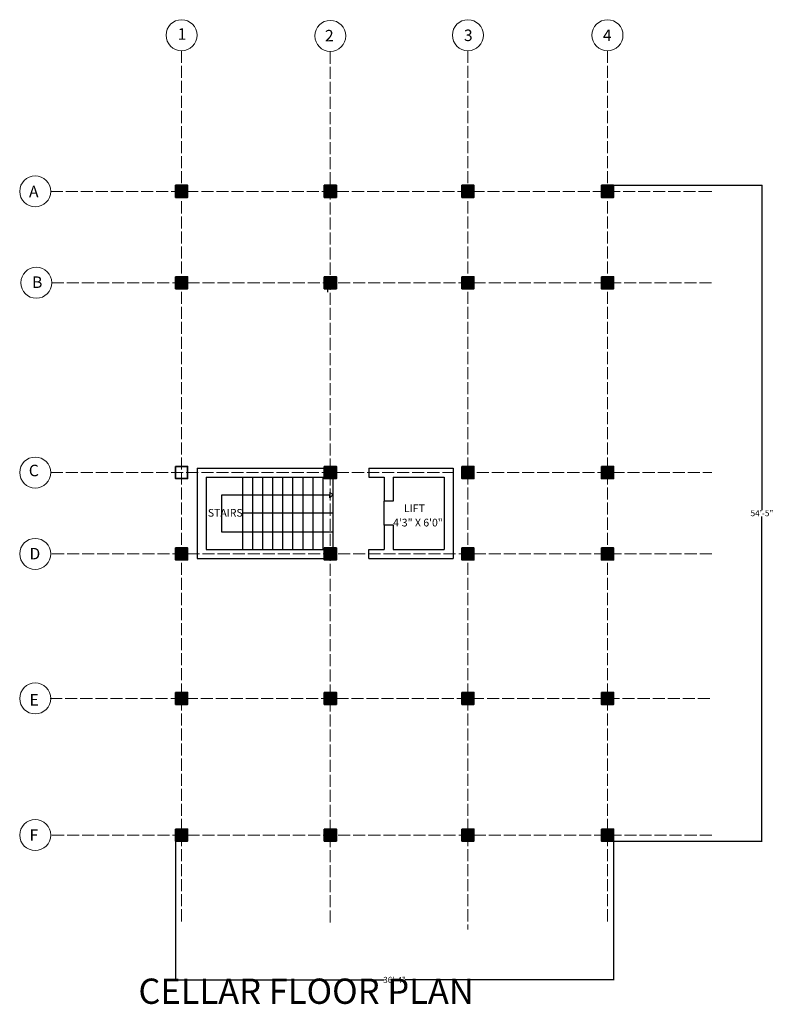
# Model space of a CAD drawing. Units: inches. Extents: x -113 to 5399, y -1393 to 3302.
# Tile 19 of 40: x 778 to 1528, y 2203 to 3184. Entities that reach past the tile are written whole.
import ezdxf

# ---------------------------------------------------------------- set-up
doc = ezdxf.new("R2010")
doc.units = ezdxf.units.IN
doc.header["$MEASUREMENT"] = 0
doc.linetypes.add('ACAD_ISO02W100', pattern=[15, 12, -3])
for name, color, linetype, lineweight in [('A-ANNO-DIMS', 254, 'Continuous', 18), ('A-ANNO-TEXT', 7, 'Continuous', 25), ('A-AREA-IDEN', 4, 'Continuous', 18), ('A-COLS', 7, 'Continuous', 35), ('A-GRID-IDEN', 7, 'Continuous', 18), ('GRIDS', 7, 'ACAD_ISO02W100', 13), ('stairs', 210, 'Continuous', 25), ('walls', 1, 'Continuous', 25)]:
    doc.layers.add(name, color=color, linetype=linetype, lineweight=lineweight)
doc.styles.get("Standard").update_dxf_attribs({"font": 'arial.ttf'})
doc.dimstyles.get("Standard").update_dxf_attribs({"dimtxt": 6, "dimasz": 0.18, "dimexe": 0.18, "dimexo": 0.0625, "dimgap": 0.09, "dimtad": 0, "dimtih": 1, "dimtoh": 1, "dimdec": 1, "dimzin": 0, "dimdsep": 46, "dimlunit": 4, "dimtxsty": 'Standard', "dimblk": 'ARCHTICK', "dimcen": 0.09, "dimadec": 0, "dimazin": 0, "dimtfac": 1, "dimtdec": 1, "dimtofl": 0, "dimtmove": 0, "dimatfit": 3, "dimfxl": 1, "dimtolj": 1, "dimtzin": 0, "dimarcsym": 0})

# ---------------------------------------------------------------- blocks, each defined once
blk = doc.blocks.new('COLUMN-12IN-SQUARE')
h = blk.add_hatch(color=256)
h.dxf.hatch_style = 1
h.paths.add_polyline_path([(6, 6), (-6, 6), (-6, -6), (6, -6)])
blk.add_lwpolyline([(-6, 6), (6, 6), (6, -6), (-6, -6)], close=True)
blk = doc.blocks.new('STAIR-CELLAR-PLAN')
for p, q in [((20.54, 72), (20.54, 0)), ((30.54, 72), (30.54, 0)), ((40.54, 72), (40.54, 0)), ((50.54, 72), (50.54, 0)), ((60.54, 72), (60.54, 0)), ((70.54, 72), (70.54, 0)), ((80.54, 72), (80.54, 0)), ((90.54, 72), (90.54, 0)), ((100.54, 72), (100.54, 0)), ((110.54, 70.5), (110.54, 1.5)), ((0, 17.09), (0, 54.14)), ((0, 54.14), (107.61, 54.14)), ((110.54, 54.14), (107.61, 56.9)), ((107.61, 56.9), (107.61, 54.14)), ((110.54, 54.14), (107.61, 51.38)), ((107.61, 51.38), (107.61, 54.14)), ((110.54, 36), (20.54, 36)), ((110.54, 17.09), (0, 17.09))]:
    blk.add_line(p, q)
blk = doc.blocks.new('GRID-BUBBLE-A')
blk.add_circle((0, 0), 15.44)
blk.add_text('A', height=11.45).set_placement((-6.15, -5.94))
blk = doc.blocks.new('GRID-BUBBLE-B')
blk.add_circle((0, 0), 15.44)
blk.add_text('B', height=11.45).set_placement((-4.23, -5.2))
blk = doc.blocks.new('GRID-BUBBLE-C')
blk.add_circle((0, 0), 15.44)
blk.add_text('C', height=11.45).set_placement((-6.38, -3.72))
blk = doc.blocks.new('GRID-BUBBLE-D')
blk.add_circle((0, 0), 15.44)
blk.add_text('D', height=11.45).set_placement((-5.69, -5.49))
blk = doc.blocks.new('GRID-BUBBLE-E')
blk.add_circle((0, 0), 15.44)
blk.add_text('E', height=11.45).set_placement((-5.69, -7.06))
blk = doc.blocks.new('GRID-BUBBLE-F')
blk.add_circle((0, 0), 15.44)
blk.add_text('F', height=11.45).set_placement((-5.69, -5.75))
blk = doc.blocks.new('GRID-BUBBLE-1')
blk.add_circle((0, 0), 15.44)
blk.add_text('1', height=11.45).set_placement((-3.99, -4.52))
blk = doc.blocks.new('GRID-BUBBLE-2')
blk.add_circle((0, 0), 15.44)
blk.add_text('2', height=11.45).set_placement((-5.33, -5.46))
blk = doc.blocks.new('GRID-BUBBLE-3')
blk.add_circle((0, 0), 15.44)
blk.add_text('3', height=11.45).set_placement((-3.95, -5.82))
blk = doc.blocks.new('GRID-BUBBLE-4')
blk.add_circle((0, 0), 15.44)
blk.add_text('4', height=11.45).set_placement((-4.57, -5.82))
blk = doc.blocks.new('_ArchTick')
at = {"color": 0, "linetype": 'ByBlock', "const_width": 0.15}
blk.add_lwpolyline([(-0.5, -0.5), (0.5, 0.5)], dxfattribs=at)
blk = doc.blocks.new('*D207')
at = {"layer": 'A-ANNO-DIMS', "color": 0, "lineweight": -2, "transparency": 16777216}
for p, q in [((932.87, 2365.95), (932.87, 2227.62)), ((1368.94, 2365.95), (1368.94, 2227.62)), ((932.87, 2227.8), (1140.51, 2227.8)), ((1368.94, 2227.8), (1161.3, 2227.8))]:
    blk.add_line(p, q, dxfattribs=at)
at = {"layer": 'Defpoints', "color": 0, "transparency": 16777216}
for p in [(932.87, 2366.02), (1368.94, 2366.02), (1368.94, 2227.8)]:
    blk.add_point(p, dxfattribs=at)
at = {"layer": 'A-ANNO-DIMS', "color": 0, "lineweight": -2, "transparency": 16777216, "xscale": 0.18, "yscale": 0.18, "zscale": 0.18, "rotation": 180}
blk.add_blockref('_ArchTick', (932.87, 2227.8), dxfattribs=at)
at = {"layer": 'A-ANNO-DIMS', "color": 0, "lineweight": -2, "transparency": 16777216, "xscale": 0.18, "yscale": 0.18, "zscale": 0.18}
blk.add_blockref('_ArchTick', (1368.94, 2227.8), dxfattribs=at)
at = {"layer": 'A-ANNO-DIMS', "color": 0, "transparency": 16777216, "insert": (1150.9, 2227.8), "char_height": 6, "attachment_point": 5}
blk.add_mtext('\\A1;36\'-4"', dxfattribs=at)
blk = doc.blocks.new('*D208')
at = {"layer": 'A-ANNO-DIMS', "color": 0, "lineweight": -2, "transparency": 16777216}
for p, q in [((1369.01, 3019.02), (1516.94, 3019.02)), ((1516.76, 3019.02), (1516.76, 2695.66)), ((1516.76, 2366.02), (1516.76, 2689.38)), ((1369.01, 2366.02), (1516.94, 2366.02))]:
    blk.add_line(p, q, dxfattribs=at)
at = {"layer": 'Defpoints', "color": 0, "transparency": 16777216}
for p in [(1368.94, 3019.02), (1516.76, 3019.02), (1368.94, 2366.02)]:
    blk.add_point(p, dxfattribs=at)
at = {"layer": 'A-ANNO-DIMS', "color": 0, "lineweight": -2, "transparency": 16777216, "xscale": 0.18, "yscale": 0.18, "zscale": 0.18}
for p, rotation in [((1516.76, 3019.02), 90), ((1516.76, 2366.02), 270)]:
    blk.add_blockref('_ArchTick', p, dxfattribs=dict(at, rotation=rotation))
at = {"layer": 'A-ANNO-DIMS', "color": 0, "transparency": 16777216, "insert": (1516.76, 2692.52), "char_height": 6, "attachment_point": 5}
blk.add_mtext('\\A1;54\'-5"', dxfattribs=at)

msp = doc.modelspace()

# ---------------------------------------------------------------- linework, layer by layer
at = {"layer": 'A-COLS'}
msp.add_lwpolyline([(932.87, 2739.02), (944.87, 2739.02), (944.87, 2727.02), (932.87, 2727.02)], close=True, dxfattribs=at)
at = {"layer": 'GRIDS'}
for p, q in [((938.87, 3153.08), (938.87, 2285.73)), ((1086.94, 2285.03), (1086.94, 3152.38)), ((1223.94, 3153.08), (1223.94, 2277.8)), ((1362.94, 3153.08), (1362.94, 2285.48)), ((808.51, 3013.02), (1457.4, 3013.02)), ((1457.4, 3013.02), (1466.76, 3013.02)), ((809.63, 2922.02), (1466.76, 2922.02)), ((808.51, 2733.02), (1209.44, 2733.02)), ((1217.94, 2733.02), (1466.76, 2733.02)), ((1466.76, 2652.02), (808.51, 2652.02)), ((807.97, 2508.02), (1466.76, 2508.02)), ((1466.76, 2372.02), (808.51, 2372.02))]:
    msp.add_line(p, q, dxfattribs=at)
at = {"layer": 'walls'}
for p, q in [((1084.44, 2912.52), (1084.44, 2924.52)), ((1084.44, 2924.52), (1089.44, 2924.52)), ((954.44, 2737.52), (1080.94, 2737.52)), ((954.44, 2737.52), (954.44, 2647.52)), ((1089.44, 2737.52), (1089.44, 2728.52)), ((1125.44, 2737.52), (1209.44, 2737.52)), ((1125.44, 2737.52), (1125.44, 2728.52)), ((1209.44, 2737.52), (1209.44, 2656.52)), ((1217.94, 2737.52), (1221.44, 2737.52)), ((963.44, 2728.52), (1080.94, 2728.52)), ((963.44, 2728.52), (963.44, 2656.52)), ((1125.44, 2728.52), (1140.44, 2728.52)), ((1140.44, 2728.52), (1140.44, 2704.52)), ((1149.44, 2728.52), (1149.44, 2704.52)), ((1149.44, 2728.52), (1200.44, 2728.52)), ((1200.44, 2728.52), (1200.44, 2656.52)), ((1217.94, 2728.52), (1226.44, 2728.52)), ((1149.44, 2704.52), (1140.44, 2704.52)), ((1140.44, 2680.52), (1140.44, 2704.52)), ((1209.44, 2688.02), (1209.44, 2647.52)), ((1140.44, 2680.52), (1140.44, 2656.52)), ((1149.44, 2680.52), (1140.44, 2680.52)), ((1149.44, 2680.52), (1149.44, 2656.52)), ((954.44, 2647.52), (1080.94, 2647.52)), ((963.44, 2656.52), (1080.94, 2656.52)), ((1089.44, 2647.52), (1089.44, 2656.52)), ((1125.44, 2656.52), (1140.44, 2656.52)), ((1125.44, 2647.52), (1125.44, 2656.52)), ((1125.44, 2647.52), (1209.44, 2647.52)), ((1149.44, 2656.52), (1200.44, 2656.52)), ((1217.94, 2656.52), (1226.44, 2656.52)), ((1217.94, 2647.52), (1221.44, 2647.52)), ((1084.44, 2505.52), (1089.44, 2505.52))]:
    msp.add_line(p, q, dxfattribs=at)

# ---------------------------------------------------------------- block references
at = {"layer": 'A-COLS'}
for p in [(938.87, 3013.02), (1086.94, 3013.02), (1223.94, 3013.02), (1362.94, 3013.02), (938.87, 2922.02), (1086.94, 2922.02), (1223.94, 2922.02), (1362.94, 2922.02), (1086.94, 2733.02), (1223.94, 2733.02), (1362.94, 2733.02), (938.87, 2652.02), (1086.94, 2652.02), (1223.94, 2652.02), (1362.94, 2652.02), (938.87, 2508.02), (1086.94, 2508.02), (1223.94, 2508.02), (1362.94, 2508.02), (938.87, 2372.02), (1086.94, 2372.02), (1223.94, 2372.02), (1362.94, 2372.02)]:
    msp.add_blockref('COLUMN-12IN-SQUARE', p, dxfattribs=at)
at = {"layer": 'A-GRID-IDEN'}
for name, p in [('GRID-BUBBLE-1', (938.87, 3168.52)), ('GRID-BUBBLE-2', (1086.94, 3167.81)), ('GRID-BUBBLE-3', (1223.94, 3168.52)), ('GRID-BUBBLE-4', (1362.94, 3168.52)), ('GRID-BUBBLE-A', (793.07, 3013.02)), ('GRID-BUBBLE-B', (794.2, 2922.02)), ('GRID-BUBBLE-C', (793.07, 2733.02)), ('GRID-BUBBLE-D', (793.07, 2652.02)), ('GRID-BUBBLE-E', (793.07, 2508.02)), ('GRID-BUBBLE-F', (793.07, 2372.02))]:
    msp.add_blockref(name, p, dxfattribs=at)
at = {"layer": 'stairs'}
msp.add_blockref('STAIR-CELLAR-PLAN', (978.9, 2656.52), dxfattribs=at)

# ---------------------------------------------------------------- texts
at = {"layer": 'A-ANNO-TEXT'}
msp.add_text('CELLAR FLOOR PLAN', height=25.17, dxfattribs=at).set_placement((895.86, 2203.91))
at = {"layer": 'A-AREA-IDEN'}
for s, height, p in [('STAIRS', 7.647, (964.99, 2689.07)), ('LIFT', 7.647, (1160.33, 2693.58)), ('4\'3" X 6\'0"', 7.6473, (1149.44, 2679.31))]:
    msp.add_text(s, height=height, dxfattribs=at).set_placement(p)

# ---------------------------------------------------------------- dimensions: what is measured, and where the dimension line sits
at = {"layer": 'A-ANNO-DIMS'}
dim = msp.add_linear_dim(base=(1516.76, 3019.02), p1=(1368.94, 2366.02), p2=(1368.94, 3019.02), angle=90, dimstyle='Standard', override={"dimdec": 1, "dimlfac": 1, "dimrnd": 0, "dimzin": 1, "dimdsep": 46, "dimlunit": 4, "dimfrac": 2}, dxfattribs=at)
dim.commit()
dim.dimension.update_dxf_attribs({"geometry": '*D208', "text_midpoint": (1516.76, 2692.52)})
dim = msp.add_linear_dim(base=(1368.94, 2227.8), p1=(932.87, 2366.02), p2=(1368.94, 2366.02), dimstyle='Standard', override={"dimdec": 1, "dimlfac": 1, "dimrnd": 0, "dimzin": 1, "dimdsep": 46, "dimlunit": 4, "dimfrac": 2}, dxfattribs=at)
dim.commit()
dim.dimension.update_dxf_attribs({"geometry": '*D207', "text_midpoint": (1150.9, 2227.8)})

doc.saveas('drawing.dxf')
